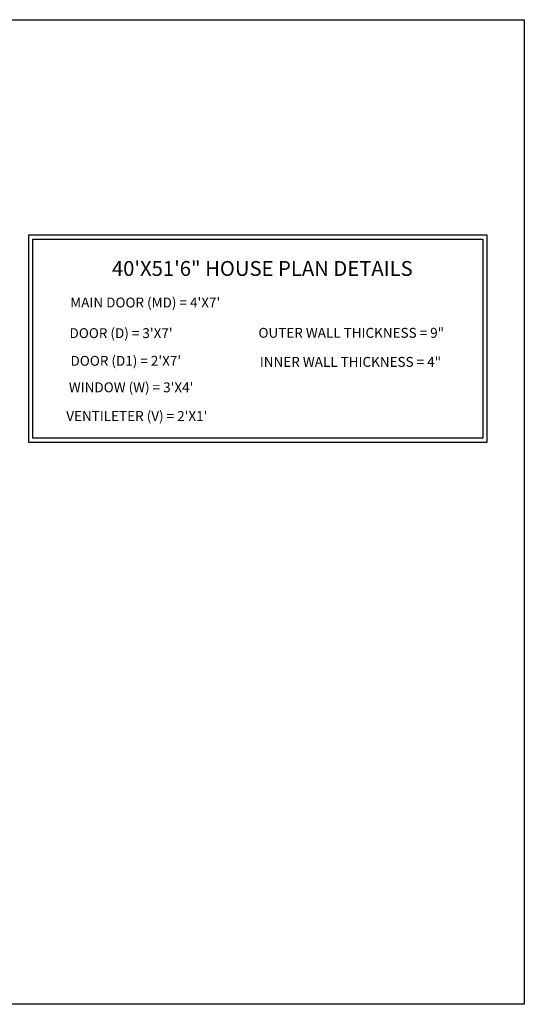
# Model space of a CAD drawing. Units: inches. Extents: x 2169 to 10664, y 1669 to 6352.
# Tile 17 of 17: x 10052 to 10664, y 5159 to 6352. Entities that reach past the tile are written whole.
import ezdxf

# ---------------------------------------------------------------- set-up
doc = ezdxf.new("R2010")
doc.units = ezdxf.units.IN
for name, color, linetype, lineweight in [('A-ANNO-TEXT', 7, 'Continuous', 18), ('A-ANNO-TITL', 3, 'Continuous', 25), ('A-ANNO-TTLB', 7, 'Continuous', 25)]:
    doc.layers.add(name, color=color, linetype=linetype, lineweight=lineweight)
doc.styles.get("Standard").update_dxf_attribs({"font": 'arial.ttf'})

msp = doc.modelspace()

# ---------------------------------------------------------------- linework, layer by layer
at = {"layer": 'A-ANNO-TTLB'}
for points in [[(9414.82, 6351.94), (10664.28, 6351.94), (10664.28, 5158.92), (9414.82, 5158.92)], [(10063.48, 6091.14), (10618.95, 6091.14), (10618.95, 5839.8), (10063.48, 5839.8)], [(10068.48, 6086.14), (10613.95, 6086.14), (10613.95, 5844.8), (10068.48, 5844.8)]]:
    msp.add_lwpolyline(points, close=True, dxfattribs=at)

# ---------------------------------------------------------------- texts
at = {"layer": 'A-ANNO-TEXT', "char_height": 12, "attachment_point": 1}
for s, width, insert in [("MAIN DOOR (MD) = 4'X7'", 1084.5311, (10113.72, 6015.26)), ("DOOR (D) = 3'X7'", 292.5215, (10112.86, 5978.14)), ('OUTER WALL THICKNESS = 9"', 296.4131, (10341.95, 5978.52)), ("DOOR (D1) = 2'X7'", 275.5147, (10114.06, 5944.6)), ('INNER WALL THICKNESS = 4"', 268.5398, (10343.58, 5943.32)), ("WINDOW (W) = 3'X4'", 276.6037, (10112.05, 5912.49)), ("VENTILETER (V) = 2'X1'", 249.0159, (10108.92, 5877.71))]:
    msp.add_mtext_dynamic_manual_height_columns(s, width=width, gutter_width=12.5, heights=[0], dxfattribs=dict(at, insert=insert))
at = {"layer": 'A-ANNO-TITL', "insert": (10164.28, 6059.5), "char_height": 18, "attachment_point": 1}
msp.add_mtext_dynamic_manual_height_columns('40\'X51\'6" HOUSE PLAN DETAILS', width=849.1663, gutter_width=12.5, heights=[0], dxfattribs=at)

doc.saveas('drawing.dxf')
